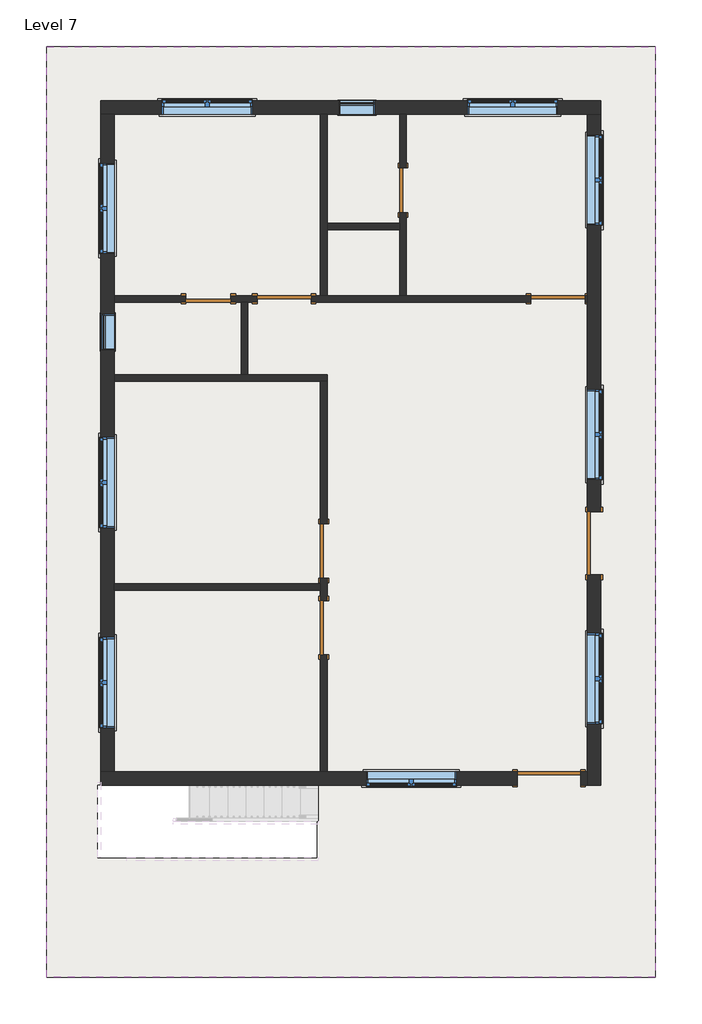
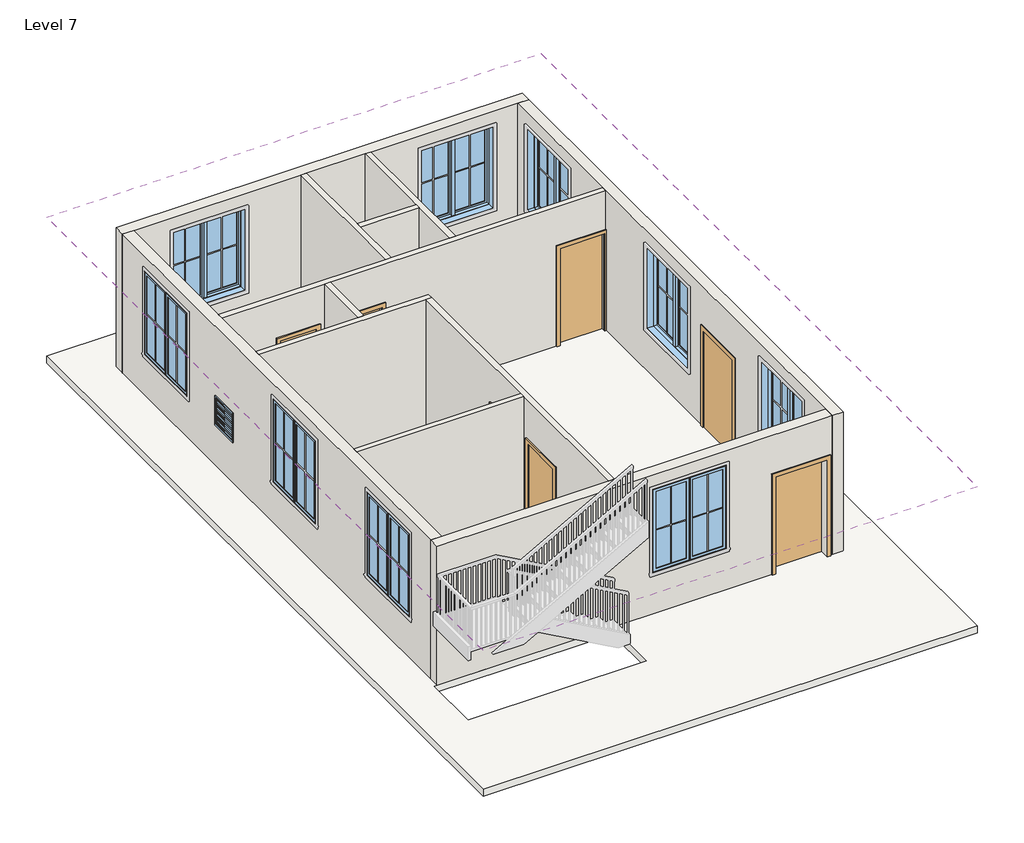
# One storey, part 1 of 3: 12 walls, 11 windows, 8 doors, 2 roofs.
"""IFC4 building model written with IfcOpenShell, lengths in millimetres."""

from ifc_helpers import new_model, si_unit, frame, origin, place, context, project, spatial, polyline, outline, extrude, faceted_brep, transform, mapped, element, save
from components import door_78caadf7, single_flush_door_3_e5f9f3c4, single_flush_door_3_305aa2a5, door_9d399b00, door_0848dd25, window_casement_double_win_5_f93960c7, window_f2d8fef0

model = new_model("IFC4")

# Units and contexts
model_context = context("Model", 3, world=origin())
ifc_project = project(units=[si_unit("LENGTHUNIT", "METRE", prefix="MILLI")], contexts=[model_context])

# Site, building, storey
site = spatial("IfcSite", under=ifc_project)
building = spatial("IfcBuilding", under=site)
storey = spatial("IfcBuildingStorey", under=building, Name="Level 7", Elevation=16002.0)

# Doors
placement = place(None, origin())
door_shape = door_78caadf7(model_context)
element("IfcDoor", 1, ObjectType="Single-Flush : DOOR 2'6\"", at=placement, inside=storey, context=model_context, shape_type="MappedRepresentation", body=[
    mapped(door_shape, transform((-377.1698569, 4707.5566963, 16002.0), x_axis=(0.0, -1.0, 0.0), y_axis=(1.0, 0.0, 0.0), z_axis=(0.0, 0.0, 1.0))),
])
element("IfcDoor", 2, ObjectType="Single-Flush : DOOR 2'6\"", at=placement, inside=storey, context=model_context, shape_type="MappedRepresentation", body=[
    mapped(door_shape, transform((-3653.7698569, 2878.7566963, 16002.0), x_axis=(1.0, 0.0, 0.0), y_axis=(0.0, 1.0, 0.0), z_axis=(0.0, 0.0, 1.0))),
])
single_flush_door_3_shape = single_flush_door_3_e5f9f3c4(model_context)
element("IfcDoor", 3, ObjectType="Single-Flush : DOOR 3'", at=placement, inside=storey, context=model_context, shape_type="MappedRepresentation", body=[
    mapped(single_flush_door_3_shape, transform((-2377.4198569, 2878.7566963, 16002.0), x_axis=(1.0, 0.0, 0.0), y_axis=(0.0, 1.0, 0.0), z_axis=(0.0, 0.0, 1.0))),
])
element("IfcDoor", 4, ObjectType="Single-Flush : DOOR 3'", at=placement, inside=storey, context=model_context, shape_type="MappedRepresentation", body=[
    mapped(single_flush_door_3_shape, transform((2232.6801431, 2878.7566963, 16002.0), x_axis=(1.0, 0.0, 0.0), y_axis=(0.0, 1.0, 0.0), z_axis=(0.0, 0.0, 1.0))),
])
element("IfcDoor", 5, ObjectType="Single-Flush : DOOR 3'", at=placement, inside=storey, context=model_context, shape_type="MappedRepresentation", body=[
    mapped(single_flush_door_3_shape, transform((-1710.6698569, -2658.4433037, 16002.0), x_axis=(0.0, 1.0, 0.0), y_axis=(-1.0, 0.0, 0.0), z_axis=(0.0, 0.0, 1.0))),
])
single_flush_door_3_2_shape = single_flush_door_3_305aa2a5(model_context)
element("IfcDoor", 6, ObjectType="Single-Flush : DOOR 3'", at=placement, inside=storey, context=model_context, shape_type="MappedRepresentation", body=[
    mapped(single_flush_door_3_2_shape, transform((-1710.6698569, -1363.0433037, 16002.0), x_axis=(0.0, -1.0, 0.0), y_axis=(1.0, 0.0, 0.0), z_axis=(0.0, 0.0, 1.0))),
])
door_2_shape = door_9d399b00(model_context)
element("IfcDoor", 7, ObjectType="Single-Flush : DOOR 3'6\"", at=placement, inside=storey, context=model_context, shape_type="MappedRepresentation", body=[
    mapped(door_2_shape, transform((2080.2801431, -5192.0933037, 16002.0), x_axis=(1.0, 0.0, 0.0), y_axis=(0.0, 1.0, 0.0), z_axis=(0.0, 0.0, 1.0))),
])
door_3_shape = door_0848dd25(model_context)
element("IfcDoor", 8, ObjectType="Single-Flush : DOOR 3'6\"", at=placement, inside=storey, context=model_context, shape_type="MappedRepresentation", body=[
    mapped(door_3_shape, transform((2842.2801431, -1236.0433037, 16002.0), x_axis=(0.0, -1.0, 0.0), y_axis=(1.0, 0.0, 0.0), z_axis=(0.0, 0.0, 1.0))),
])

# Roofs
element("IfcRoof", 9, ObjectType="ROOF 6\"", at=placement, inside=storey, context=model_context, shape_type="SweptSolid", body=[
    extrude(outline(polyline([(-6377.9198569, -8544.8933037), (-6377.9198569, 7126.9066963), (3870.9801431, 7126.9066963), (3870.9801431, -8544.8933037), (-6377.9198569, -8544.8933037)]), holes=[polyline([(-5514.3198569, -5306.3933037), (-5514.3198569, -6525.5933037), (-1831.3198569, -6525.5933037), (-1831.3198569, -5306.3933037), (-5514.3198569, -5306.3933037)])]), frame((0.0, 0.0, 15849.6), z_axis=(0.0, 0.0, 1.0), x_axis=(1.0, 0.0, 0.0)), (0.0, 0.0, 1.0), 152.4),
])
element("IfcRoof", 10, ObjectType="ROOF 6\"", at=placement, inside=storey, context=model_context, shape_type="SweptSolid", body=[
    extrude(outline(polyline([(-6377.9198569, -8544.8933037), (-6377.9198569, 7126.9066963), (3870.9801431, 7126.9066963), (3870.9801431, -8544.8933037), (-6377.9198569, -8544.8933037)]), holes=[polyline([(-5514.3198569, -5306.3933037), (-5514.3198569, -6525.5933037), (-1831.3198569, -6525.5933037), (-1831.3198569, -5306.3933037), (-5514.3198569, -5306.3933037)])]), frame((0.0, 0.0, 19050.0), z_axis=(0.0, 0.0, 1.0), x_axis=(1.0, 0.0, 0.0)), (0.0, 0.0, 1.0), 152.4),
])

# Walls
element("IfcWall", 11, ObjectType="WALL 4.5\"", at=placement, inside=storey, context=model_context, shape_type="Brep", body=[
    faceted_brep([(2689.8801431, 2821.6066963, 18135.6), (2689.8801431, 2821.6066963, 16002.0), (2727.9801431, 2821.6066963, 16002.0), (2727.9801431, 2821.6066963, 19050.0), (-2987.0198569, 2821.6066963, 19050.0), (-3101.3198569, 2821.6066963, 19050.0), (-5234.9198569, 2821.6066963, 19050.0), (-5234.9198569, 2821.6066963, 16002.0), (-4034.7698569, 2821.6066963, 16002.0), (-4034.7698569, 2821.6066963, 18135.6), (-3272.7698569, 2821.6066963, 18135.6), (-3272.7698569, 2821.6066963, 16002.0), (-3101.3198569, 2821.6066963, 16002.0), (-2987.0198569, 2821.6066963, 16002.0), (-2834.6198569, 2821.6066963, 16002.0), (-2834.6198569, 2821.6066963, 18135.6), (-1920.2198569, 2821.6066963, 18135.6), (-1920.2198569, 2821.6066963, 16002.0), (1775.4801431, 2821.6066963, 16002.0), (1775.4801431, 2821.6066963, 18135.6), (2727.9801431, 2935.9066963, 16002.0), (2689.8801431, 2935.9066963, 16002.0), (2689.8801431, 2935.9066963, 18135.6), (1775.4801431, 2935.9066963, 18135.6), (1775.4801431, 2935.9066963, 16002.0), (-320.0198569, 2935.9066963, 16002.0), (-434.3198569, 2935.9066963, 16002.0), (-1653.5198569, 2935.9066963, 16002.0), (-1767.8198569, 2935.9066963, 16002.0), (-1920.2198569, 2935.9066963, 16002.0), (-1920.2198569, 2935.9066963, 18135.6), (-2834.6198569, 2935.9066963, 18135.6), (-2834.6198569, 2935.9066963, 16002.0), (-3272.7698569, 2935.9066963, 16002.0), (-3272.7698569, 2935.9066963, 18135.6), (-4034.7698569, 2935.9066963, 18135.6), (-4034.7698569, 2935.9066963, 16002.0), (-5234.9198569, 2935.9066963, 16002.0), (-5234.9198569, 2935.9066963, 19050.0), (-1767.8198569, 2935.9066963, 19050.0), (-1653.5198569, 2935.9066963, 19050.0), (-434.3198569, 2935.9066963, 19050.0), (-320.0198569, 2935.9066963, 19050.0), (2727.9801431, 2935.9066963, 19050.0)], [[[0, 1, 2, 3, 4, 5, 6, 7, 8, 9, 10, 11, 12, 13, 14, 15, 16, 17, 18, 19]], [[20, 21, 22, 23, 24, 25, 26, 27, 28, 29, 30, 31, 32, 33, 34, 35, 36, 37, 38, 39, 40, 41, 42, 43]], [[8, 7, 37, 36]], [[14, 13, 12, 11, 33, 32]], [[18, 17, 29, 28, 27, 26, 25, 24]], [[2, 1, 21, 20]], [[3, 2, 20, 43]], [[7, 6, 38, 37]], [[34, 33, 11, 10]], [[35, 34, 10, 9]], [[36, 35, 9, 8]], [[30, 29, 17, 16]], [[31, 30, 16, 15]], [[32, 31, 15, 14]], [[22, 21, 1, 0]], [[23, 22, 0, 19]], [[24, 23, 19, 18]], [[6, 5, 4, 3, 43, 42, 41, 40, 39, 38]]]),
])
element("IfcWall", 12, ObjectType="WALL 4.5\"", at=placement, inside=storey, context=model_context, shape_type="Brep", body=[
    faceted_brep([(-1767.8198569, 5983.9066963, 16002.0), (-1767.8198569, 2935.9066963, 16002.0), (-1767.8198569, 2935.9066963, 19050.0), (-1767.8198569, 5983.9066963, 19050.0), (-1653.5198569, 5983.9066963, 16002.0), (-1653.5198569, 5983.9066963, 19050.0), (-1653.5198569, 4155.1066963, 19050.0), (-1653.5198569, 4040.8066963, 19050.0), (-1653.5198569, 2935.9066963, 19050.0), (-1653.5198569, 2935.9066963, 16002.0), (-1653.5198569, 4040.8066963, 16002.0), (-1653.5198569, 4155.1066963, 16002.0)], [[[0, 1, 2, 3]], [[4, 5, 6, 7, 8, 9, 10, 11]], [[1, 0, 4, 11, 10, 9]], [[0, 3, 5, 4]], [[2, 1, 9, 8]], [[3, 2, 8, 7, 6, 5]]]),
])
element("IfcWall", 13, ObjectType="WALL 4.5\"", at=placement, inside=storey, context=model_context, shape_type="Brep", body=[
    faceted_brep([(-320.0198569, 2935.9066963, 16002.0), (-320.0198569, 4326.5566963, 16002.0), (-320.0198569, 4326.5566963, 18135.6), (-320.0198569, 5088.5566963, 18135.6), (-320.0198569, 5088.5566963, 16002.0), (-320.0198569, 5983.9066963, 16002.0), (-320.0198569, 5983.9066963, 19050.0), (-320.0198569, 2935.9066963, 19050.0), (-434.3198569, 4326.5566963, 18135.6), (-434.3198569, 4326.5566963, 16002.0), (-434.3198569, 4155.1066963, 16002.0), (-434.3198569, 4040.8066963, 16002.0), (-434.3198569, 2935.9066963, 16002.0), (-434.3198569, 2935.9066963, 19050.0), (-434.3198569, 4040.8066963, 19050.0), (-434.3198569, 4155.1066963, 19050.0), (-434.3198569, 5983.9066963, 19050.0), (-434.3198569, 5983.9066963, 16002.0), (-434.3198569, 5088.5566963, 16002.0), (-434.3198569, 5088.5566963, 18135.6)], [[[0, 1, 2, 3, 4, 5, 6, 7]], [[8, 9, 10, 11, 12, 13, 14, 15, 16, 17, 18, 19]], [[18, 17, 5, 4]], [[12, 11, 10, 9, 1, 0]], [[6, 5, 17, 16]], [[0, 7, 13, 12]], [[2, 1, 9, 8]], [[3, 2, 8, 19]], [[4, 3, 19, 18]], [[7, 6, 16, 15, 14, 13]]]),
])
element("IfcWall", 14, ObjectType="WALL 4.5\"", at=placement, inside=storey, context=model_context, shape_type="SweptSolid", body=[
    extrude(outline(polyline([(-434.3198569, 4040.8066963), (-1653.5198569, 4040.8066963), (-1653.5198569, 4155.1066963), (-434.3198569, 4155.1066963), (-434.3198569, 4040.8066963)])), frame((0.0, 0.0, 16002.0), z_axis=(0.0, 0.0, 1.0), x_axis=(1.0, 0.0, 0.0)), (0.0, 0.0, 1.0), 3048.0),
])
element("IfcWall", 15, ObjectType="WALL 4.5\"", at=placement, inside=storey, context=model_context, shape_type="Brep", body=[
    faceted_brep([(-5234.9198569, 1488.1066963, 16002.0), (-1767.8198569, 1488.1066963, 16002.0), (-1653.5198569, 1488.1066963, 16002.0), (-1653.5198569, 1488.1066963, 19050.0), (-1767.8198569, 1488.1066963, 19050.0), (-5234.9198569, 1488.1066963, 19050.0), (-5234.9198569, 1602.4066963, 16002.0), (-5234.9198569, 1602.4066963, 19050.0), (-3101.3198569, 1602.4066963, 19050.0), (-2987.0198569, 1602.4066963, 19050.0), (-1653.5198569, 1602.4066963, 19050.0), (-1653.5198569, 1602.4066963, 16002.0), (-2987.0198569, 1602.4066963, 16002.0), (-3101.3198569, 1602.4066963, 16002.0)], [[[0, 1, 2, 3, 4, 5]], [[6, 7, 8, 9, 10, 11, 12, 13]], [[2, 1, 0, 6, 13, 12, 11]], [[0, 5, 7, 6]], [[3, 2, 11, 10]], [[5, 4, 3, 10, 9, 8, 7]]]),
])
element("IfcWall", 16, ObjectType="WALL 4.5\"", at=placement, inside=storey, context=model_context, shape_type="Brep", body=[
    faceted_brep([(-1767.8198569, -1820.2433037, 16002.0), (-1767.8198569, -1915.4933037, 16002.0), (-1767.8198569, -2029.7933037, 16002.0), (-1767.8198569, -2201.2433037, 16002.0), (-1767.8198569, -2201.2433037, 18135.6), (-1767.8198569, -3115.6433037, 18135.6), (-1767.8198569, -3115.6433037, 16002.0), (-1767.8198569, -5077.7933037, 16002.0), (-1767.8198569, -5077.7933037, 19050.0), (-1767.8198569, -2029.7933037, 19050.0), (-1767.8198569, -1915.4933037, 19050.0), (-1767.8198569, 1488.1066963, 19050.0), (-1767.8198569, 1488.1066963, 16002.0), (-1767.8198569, -905.8433037, 16002.0), (-1767.8198569, -905.8433037, 18135.6), (-1767.8198569, -1820.2433037, 18135.6), (-1653.5198569, -2201.2433037, 18135.6), (-1653.5198569, -2201.2433037, 16002.0), (-1653.5198569, -1820.2433037, 16002.0), (-1653.5198569, -1820.2433037, 18135.6), (-1653.5198569, -905.8433037, 18135.6), (-1653.5198569, -905.8433037, 16002.0), (-1653.5198569, 1488.1066963, 16002.0), (-1653.5198569, 1488.1066963, 19050.0), (-1653.5198569, -5077.7933037, 19050.0), (-1653.5198569, -5077.7933037, 16002.0), (-1653.5198569, -3115.6433037, 16002.0), (-1653.5198569, -3115.6433037, 18135.6)], [[[0, 1, 2, 3, 4, 5, 6, 7, 8, 9, 10, 11, 12, 13, 14, 15]], [[16, 17, 18, 19, 20, 21, 22, 23, 24, 25, 26, 27]], [[13, 12, 22, 21]], [[26, 25, 7, 6]], [[18, 17, 3, 2, 1, 0]], [[12, 11, 23, 22]], [[8, 7, 25, 24]], [[19, 18, 0, 15]], [[20, 19, 15, 14]], [[21, 20, 14, 13]], [[4, 3, 17, 16]], [[5, 4, 16, 27]], [[6, 5, 27, 26]], [[11, 10, 9, 8, 24, 23]]]),
])
element("IfcWall", 17, ObjectType="WALL 4.5\"", at=placement, inside=storey, context=model_context, shape_type="SweptSolid", body=[
    extrude(outline(polyline([(-1767.8198569, -2029.7933037), (-5234.9198569, -2029.7933037), (-5234.9198569, -1915.4933037), (-1767.8198569, -1915.4933037), (-1767.8198569, -2029.7933037)])), frame((0.0, 0.0, 16002.0), z_axis=(0.0, 0.0, 1.0), x_axis=(1.0, 0.0, 0.0)), (0.0, 0.0, 1.0), 3048.0),
])
element("IfcWall", 18, ObjectType="WALL 4.5\"", at=placement, inside=storey, context=model_context, shape_type="SweptSolid", body=[
    extrude(outline(polyline([(-3101.3198569, 1602.4066963), (-3101.3198569, 2821.6066963), (-2987.0198569, 2821.6066963), (-2987.0198569, 1602.4066963), (-3101.3198569, 1602.4066963)])), frame((0.0, 0.0, 16002.0), z_axis=(0.0, 0.0, 1.0), x_axis=(1.0, 0.0, 0.0)), (0.0, 0.0, 1.0), 3048.0),
])
element("IfcWall", 19, ObjectType="WALL 9\"", at=placement, inside=storey, context=model_context, shape_type="Brep", body=[
    faceted_brep([(-5463.5198569, 5983.9066963, 16002.0), (-5234.9198569, 5983.9066963, 16002.0), (-1767.8198569, 5983.9066963, 16002.0), (-1653.5198569, 5983.9066963, 16002.0), (-434.3198569, 5983.9066963, 16002.0), (-320.0198569, 5983.9066963, 16002.0), (2727.9801431, 5983.9066963, 16002.0), (2956.5801431, 5983.9066963, 16002.0), (2956.5801431, 5983.9066963, 19050.0), (2727.9801431, 5983.9066963, 19050.0), (-320.0198569, 5983.9066963, 19050.0), (-434.3198569, 5983.9066963, 19050.0), (-1653.5198569, 5983.9066963, 19050.0), (-1767.8198569, 5983.9066963, 19050.0), (-5234.9198569, 5983.9066963, 19050.0), (-5463.5198569, 5983.9066963, 19050.0), (2232.6801431, 5983.9066963, 18745.2), (2232.6801431, 5983.9066963, 16916.4), (708.6801431, 5983.9066963, 16916.4), (708.6801431, 5983.9066963, 18745.2), (-2910.8198569, 5983.9066963, 18745.2), (-2910.8198569, 5983.9066963, 16916.4), (-4434.8198569, 5983.9066963, 16916.4), (-4434.8198569, 5983.9066963, 18745.2), (-1456.6698569, 5983.9066963, 17526.0), (-847.0698569, 5983.9066963, 17526.0), (-847.0698569, 5983.9066963, 16916.4), (-1456.6698569, 5983.9066963, 16916.4), (-5463.5198569, 6212.5066963, 16002.0), (-5463.5198569, 6212.5066963, 19050.0), (2956.5801431, 6212.5066963, 19050.0), (2956.5801431, 6212.5066963, 16002.0), (2232.6801431, 6212.5066963, 18745.2), (708.6801431, 6212.5066963, 18745.2), (708.6801431, 6212.5066963, 16916.4), (2232.6801431, 6212.5066963, 16916.4), (-2910.8198569, 6212.5066963, 18745.2), (-4434.8198569, 6212.5066963, 18745.2), (-4434.8198569, 6212.5066963, 16916.4), (-2910.8198569, 6212.5066963, 16916.4), (-1456.6698569, 6212.5066963, 17526.0), (-1456.6698569, 6212.5066963, 16916.4), (-847.0698569, 6212.5066963, 16916.4), (-847.0698569, 6212.5066963, 17526.0)], [[[0, 1, 2, 3, 4, 5, 6, 7, 8, 9, 10, 11, 12, 13, 14, 15], [16, 17, 18, 19], [20, 21, 22, 23], [24, 25, 26, 27]], [[28, 29, 30, 31], [32, 33, 34, 35], [36, 37, 38, 39], [40, 41, 42, 43]], [[7, 6, 5, 4, 3, 2, 1, 0, 28, 31]], [[8, 7, 31, 30]], [[0, 15, 29, 28]], [[17, 16, 32, 35]], [[18, 17, 35, 34]], [[19, 18, 34, 33]], [[16, 19, 33, 32]], [[21, 20, 36, 39]], [[22, 21, 39, 38]], [[23, 22, 38, 37]], [[20, 23, 37, 36]], [[41, 40, 24, 27]], [[42, 41, 27, 26]], [[43, 42, 26, 25]], [[40, 43, 25, 24]], [[15, 14, 13, 12, 11, 10, 9, 8, 30, 29]]]),
])
element("IfcWall", 20, ObjectType="WALL 9\"", at=placement, inside=storey, context=model_context, shape_type="Brep", body=[
    faceted_brep([(2727.9801431, -1769.4433037, 18135.6), (2727.9801431, -1769.4433037, 16002.0), (2727.9801431, -5077.7933037, 16002.0), (2727.9801431, -5306.3933037, 16002.0), (2727.9801431, -5306.3933037, 19050.0), (2727.9801431, -5077.7933037, 19050.0), (2727.9801431, 2821.6066963, 19050.0), (2727.9801431, 2935.9066963, 19050.0), (2727.9801431, 5983.9066963, 19050.0), (2727.9801431, 5983.9066963, 16002.0), (2727.9801431, 2935.9066963, 16002.0), (2727.9801431, 2821.6066963, 16002.0), (2727.9801431, -702.6433037, 16002.0), (2727.9801431, -702.6433037, 18135.6), (2727.9801431, 4117.0066963, 18745.2), (2727.9801431, 4117.0066963, 16916.4), (2727.9801431, 5641.0066963, 16916.4), (2727.9801431, 5641.0066963, 18745.2), (2727.9801431, -169.2433037, 18745.2), (2727.9801431, -169.2433037, 16916.4), (2727.9801431, 1354.7566963, 16916.4), (2727.9801431, 1354.7566963, 18745.2), (2727.9801431, -4277.6933037, 18745.2), (2727.9801431, -4277.6933037, 16916.4), (2727.9801431, -2753.6933037, 16916.4), (2727.9801431, -2753.6933037, 18745.2), (2956.5801431, -5306.3933037, 16002.0), (2956.5801431, -1769.4433037, 16002.0), (2956.5801431, -1769.4433037, 18135.6), (2956.5801431, -702.6433037, 18135.6), (2956.5801431, -702.6433037, 16002.0), (2956.5801431, 5983.9066963, 16002.0), (2956.5801431, 5983.9066963, 19050.0), (2956.5801431, -5306.3933037, 19050.0), (2956.5801431, 4117.0066963, 18745.2), (2956.5801431, 5641.0066963, 18745.2), (2956.5801431, 5641.0066963, 16916.4), (2956.5801431, 4117.0066963, 16916.4), (2956.5801431, -169.2433037, 18745.2), (2956.5801431, 1354.7566963, 18745.2), (2956.5801431, 1354.7566963, 16916.4), (2956.5801431, -169.2433037, 16916.4), (2956.5801431, -4277.6933037, 18745.2), (2956.5801431, -2753.6933037, 18745.2), (2956.5801431, -2753.6933037, 16916.4), (2956.5801431, -4277.6933037, 16916.4)], [[[0, 1, 2, 3, 4, 5, 6, 7, 8, 9, 10, 11, 12, 13], [14, 15, 16, 17], [18, 19, 20, 21], [22, 23, 24, 25]], [[26, 27, 28, 29, 30, 31, 32, 33], [34, 35, 36, 37], [38, 39, 40, 41], [42, 43, 44, 45]], [[3, 2, 1, 27, 26]], [[12, 11, 10, 9, 31, 30]], [[9, 8, 32, 31]], [[4, 3, 26, 33]], [[15, 14, 34, 37]], [[16, 15, 37, 36]], [[17, 16, 36, 35]], [[14, 17, 35, 34]], [[19, 18, 38, 41]], [[20, 19, 41, 40]], [[21, 20, 40, 39]], [[18, 21, 39, 38]], [[23, 22, 42, 45]], [[24, 23, 45, 44]], [[25, 24, 44, 43]], [[22, 25, 43, 42]], [[28, 27, 1, 0]], [[29, 28, 0, 13]], [[30, 29, 13, 12]], [[8, 7, 6, 5, 4, 33, 32]]]),
])
element("IfcWall", 21, ObjectType="WALL 9\"", at=placement, inside=storey, context=model_context, shape_type="Brep", body=[
    faceted_brep([(2727.9801431, -5077.7933037, 16002.0), (2613.6801431, -5077.7933037, 16002.0), (2613.6801431, -5077.7933037, 18135.6), (1546.8801431, -5077.7933037, 18135.6), (1546.8801431, -5077.7933037, 16002.0), (-1653.5198569, -5077.7933037, 16002.0), (-1767.8198569, -5077.7933037, 16002.0), (-5234.9198569, -5077.7933037, 16002.0), (-5463.5198569, -5077.7933037, 16002.0), (-5463.5198569, -5077.7933037, 19050.0), (-5234.9198569, -5077.7933037, 19050.0), (-1767.8198569, -5077.7933037, 19050.0), (-1653.5198569, -5077.7933037, 19050.0), (2727.9801431, -5077.7933037, 19050.0), (-999.4698569, -5077.7933037, 18745.2), (-999.4698569, -5077.7933037, 16916.4), (524.5301431, -5077.7933037, 16916.4), (524.5301431, -5077.7933037, 18745.2), (2613.6801431, -5306.3933037, 18135.6), (2613.6801431, -5306.3933037, 16002.0), (2727.9801431, -5306.3933037, 16002.0), (2727.9801431, -5306.3933037, 19050.0), (-1831.3198569, -5306.3933037, 19050.0), (-5463.5198569, -5306.3933037, 19050.0), (-5463.5198569, -5306.3933037, 16002.0), (1546.8801431, -5306.3933037, 16002.0), (1546.8801431, -5306.3933037, 18135.6), (-999.4698569, -5306.3933037, 18745.2), (524.5301431, -5306.3933037, 18745.2), (524.5301431, -5306.3933037, 16916.4), (-999.4698569, -5306.3933037, 16916.4)], [[[0, 1, 2, 3, 4, 5, 6, 7, 8, 9, 10, 11, 12, 13], [14, 15, 16, 17]], [[18, 19, 20, 21, 22, 23, 24, 25, 26], [27, 28, 29, 30]], [[25, 24, 8, 7, 6, 5, 4]], [[20, 19, 1, 0]], [[0, 13, 21, 20]], [[9, 8, 24, 23]], [[15, 14, 27, 30]], [[16, 15, 30, 29]], [[17, 16, 29, 28]], [[14, 17, 28, 27]], [[2, 1, 19, 18]], [[3, 2, 18, 26]], [[4, 3, 26, 25]], [[13, 12, 11, 10, 9, 23, 22, 21]]]),
])
element("IfcWall", 22, ObjectType="WALL 9\"", at=placement, inside=storey, context=model_context, shape_type="Brep", body=[
    faceted_brep([(-5234.9198569, -5077.7933037, 16002.0), (-5234.9198569, -2029.7933037, 16002.0), (-5234.9198569, -1915.4933037, 16002.0), (-5234.9198569, 1488.1066963, 16002.0), (-5234.9198569, 1602.4066963, 16002.0), (-5234.9198569, 2821.6066963, 16002.0), (-5234.9198569, 2935.9066963, 16002.0), (-5234.9198569, 5983.9066963, 16002.0), (-5234.9198569, 5983.9066963, 19050.0), (-5234.9198569, 2935.9066963, 19050.0), (-5234.9198569, 2821.6066963, 19050.0), (-5234.9198569, 1602.4066963, 19050.0), (-5234.9198569, 1488.1066963, 19050.0), (-5234.9198569, -1915.4933037, 19050.0), (-5234.9198569, -2029.7933037, 19050.0), (-5234.9198569, -5077.7933037, 19050.0), (-5234.9198569, -2820.3683037, 18745.2), (-5234.9198569, -2820.3683037, 16916.4), (-5234.9198569, -4344.3683037, 16916.4), (-5234.9198569, -4344.3683037, 18745.2), (-5234.9198569, 548.3066963, 18745.2), (-5234.9198569, 548.3066963, 16916.4), (-5234.9198569, -975.6933037, 16916.4), (-5234.9198569, -975.6933037, 18745.2), (-5234.9198569, 5164.7566963, 18745.2), (-5234.9198569, 5164.7566963, 16916.4), (-5234.9198569, 3640.7566963, 16916.4), (-5234.9198569, 3640.7566963, 18745.2), (-5234.9198569, 2015.1566963, 17526.0), (-5234.9198569, 2624.7566963, 17526.0), (-5234.9198569, 2624.7566963, 16916.4), (-5234.9198569, 2015.1566963, 16916.4), (-5463.5198569, -5077.7933037, 16002.0), (-5463.5198569, -5077.7933037, 19050.0), (-5463.5198569, 5983.9066963, 19050.0), (-5463.5198569, 5983.9066963, 16002.0), (-5463.5198569, -2820.3683037, 18745.2), (-5463.5198569, -4344.3683037, 18745.2), (-5463.5198569, -4344.3683037, 16916.4), (-5463.5198569, -2820.3683037, 16916.4), (-5463.5198569, 548.3066963, 18745.2), (-5463.5198569, -975.6933037, 18745.2), (-5463.5198569, -975.6933037, 16916.4), (-5463.5198569, 548.3066963, 16916.4), (-5463.5198569, 5164.7566963, 18745.2), (-5463.5198569, 3640.7566963, 18745.2), (-5463.5198569, 3640.7566963, 16916.4), (-5463.5198569, 5164.7566963, 16916.4), (-5463.5198569, 2015.1566963, 17526.0), (-5463.5198569, 2015.1566963, 16916.4), (-5463.5198569, 2624.7566963, 16916.4), (-5463.5198569, 2624.7566963, 17526.0)], [[[0, 1, 2, 3, 4, 5, 6, 7, 8, 9, 10, 11, 12, 13, 14, 15], [16, 17, 18, 19], [20, 21, 22, 23], [24, 25, 26, 27], [28, 29, 30, 31]], [[32, 33, 34, 35], [36, 37, 38, 39], [40, 41, 42, 43], [44, 45, 46, 47], [48, 49, 50, 51]], [[7, 6, 5, 4, 3, 2, 1, 0, 32, 35]], [[8, 7, 35, 34]], [[0, 15, 33, 32]], [[17, 16, 36, 39]], [[18, 17, 39, 38]], [[19, 18, 38, 37]], [[16, 19, 37, 36]], [[21, 20, 40, 43]], [[22, 21, 43, 42]], [[23, 22, 42, 41]], [[20, 23, 41, 40]], [[25, 24, 44, 47]], [[26, 25, 47, 46]], [[27, 26, 46, 45]], [[24, 27, 45, 44]], [[49, 48, 28, 31]], [[50, 49, 31, 30]], [[51, 50, 30, 29]], [[48, 51, 29, 28]], [[15, 14, 13, 12, 11, 10, 9, 8, 34, 33]]]),
])

# Windows
window_casement_double_win_5_shape = window_casement_double_win_5_f93960c7(model_context)
element("IfcWindow", 23, ObjectType="Window-Casement-Double : WIN 5'", at=placement, inside=storey, context=model_context, shape_type="MappedRepresentation", body=[
    mapped(window_casement_double_win_5_shape, transform((-5349.2198569, -3582.3683037, 16002.0), x_axis=(0.0, 1.0, 0.0), y_axis=(-1.0, 0.0, 0.0), z_axis=(0.0, 0.0, 1.0))),
])
element("IfcWindow", 24, ObjectType="Window-Casement-Double : WIN 5'", at=placement, inside=storey, context=model_context, shape_type="MappedRepresentation", body=[
    mapped(window_casement_double_win_5_shape, transform((-5349.2198569, -213.6933037, 16002.0), x_axis=(0.0, 1.0, 0.0), y_axis=(-1.0, 0.0, 0.0), z_axis=(0.0, 0.0, 1.0))),
])
element("IfcWindow", 25, ObjectType="Window-Casement-Double : WIN 5'", at=placement, inside=storey, context=model_context, shape_type="MappedRepresentation", body=[
    mapped(window_casement_double_win_5_shape, transform((-5349.2198569, 4402.7566963, 16002.0), x_axis=(0.0, 1.0, 0.0), y_axis=(-1.0, 0.0, 0.0), z_axis=(0.0, 0.0, 1.0))),
])
element("IfcWindow", 26, ObjectType="Window-Casement-Double : WIN 5'", at=placement, inside=storey, context=model_context, shape_type="MappedRepresentation", body=[
    mapped(window_casement_double_win_5_shape, transform((2842.2801431, 4879.0066963, 16002.0), x_axis=(0.0, -1.0, 0.0), y_axis=(1.0, 0.0, 0.0), z_axis=(0.0, 0.0, 1.0))),
])
element("IfcWindow", 27, ObjectType="Window-Casement-Double : WIN 5'", at=placement, inside=storey, context=model_context, shape_type="MappedRepresentation", body=[
    mapped(window_casement_double_win_5_shape, transform((2842.2801431, 592.7566963, 16002.0), x_axis=(0.0, -1.0, 0.0), y_axis=(1.0, 0.0, 0.0), z_axis=(0.0, 0.0, 1.0))),
])
element("IfcWindow", 28, ObjectType="Window-Casement-Double : WIN 5'", at=placement, inside=storey, context=model_context, shape_type="MappedRepresentation", body=[
    mapped(window_casement_double_win_5_shape, transform((2842.2801431, -3515.6933037, 16002.0), x_axis=(0.0, -1.0, 0.0), y_axis=(1.0, 0.0, 0.0), z_axis=(0.0, 0.0, 1.0))),
])
element("IfcWindow", 29, ObjectType="Window-Casement-Double : WIN 5'", at=placement, inside=storey, context=model_context, shape_type="MappedRepresentation", body=[
    mapped(window_casement_double_win_5_shape, transform((-237.4698569, -5192.0933037, 16002.0), x_axis=(-1.0, 0.0, 0.0), y_axis=(0.0, -1.0, 0.0), z_axis=(0.0, 0.0, 1.0))),
])
element("IfcWindow", 30, ObjectType="Window-Casement-Double : WIN 5'", at=placement, inside=storey, context=model_context, shape_type="MappedRepresentation", body=[
    mapped(window_casement_double_win_5_shape, transform((1470.6801431, 6098.2066963, 16002.0), x_axis=(1.0, 0.0, 0.0), y_axis=(0.0, 1.0, 0.0), z_axis=(0.0, 0.0, 1.0))),
])
element("IfcWindow", 31, ObjectType="Window-Casement-Double : WIN 5'", at=placement, inside=storey, context=model_context, shape_type="MappedRepresentation", body=[
    mapped(window_casement_double_win_5_shape, transform((-3672.8198569, 6098.2066963, 16002.0), x_axis=(1.0, 0.0, 0.0), y_axis=(0.0, 1.0, 0.0), z_axis=(0.0, 0.0, 1.0))),
])
window_shape = window_f2d8fef0(model_context)
element("IfcWindow", 32, ObjectType="Window-Louvers : 24\" x 24\"", at=placement, inside=storey, context=model_context, shape_type="MappedRepresentation", body=[
    mapped(window_shape, transform((-1151.8698569, 6104.5566963, 16002.0), x_axis=(1.0, 0.0, 0.0), y_axis=(0.0, 1.0, 0.0), z_axis=(0.0, 0.0, 1.0))),
])
element("IfcWindow", 33, ObjectType="Window-Louvers : 24\" x 24\"", at=placement, inside=storey, context=model_context, shape_type="MappedRepresentation", body=[
    mapped(window_shape, transform((-5355.5698569, 2319.9566963, 16002.0), x_axis=(0.0, 1.0, 0.0), y_axis=(-1.0, 0.0, 0.0), z_axis=(0.0, 0.0, 1.0))),
])

save(model, "model.ifc")

# Revit data of these elements
# Type "Single-Flush : DOOR 2'6\""
#   Type Mark = "10"
#   Construction Type Id = "MDOOR"
#   Assembly Code = "C1020"
#   Analytic Construction = "Metal"
#   Thickness = 0' - 2"
#   Heat Transfer Coefficient (U) = 0.651978 BTU/(h·ft²·°F)
#   Height = 7' - 0"
#   Trim Projection Ext = 0' - 1"
#   Trim Projection Int = 0' - 1"
#   Trim Width = 0' - 3"
#   Width = 2' - 6"
#   Define Thermal Properties by = 1
#   Door Material = Door - Panel
#   Frame Material = Door - Frame
#   Visual Light Transmittance = 0
#   Solar Heat Gain Coefficient = 0
#   Function = (empty or 0)
#   Wall Closure = (empty or 0)
# Type "Single-Flush : DOOR 3'"
#   Type Mark = "8"
#   Construction Type Id = "MDOOR"
#   Assembly Code = "C1020"
#   Analytic Construction = "Metal"
#   Thickness = 0' - 2"
#   Heat Transfer Coefficient (U) = 0.651978 BTU/(h·ft²·°F)
#   Height = 7' - 0"
#   Trim Projection Ext = 0' - 1"
#   Trim Projection Int = 0' - 1"
#   Trim Width = 0' - 3"
#   Width = 3' - 0"
#   Define Thermal Properties by = 1
#   Door Material = Door - Panel
#   Frame Material = Door - Frame
#   Visual Light Transmittance = 0
#   Solar Heat Gain Coefficient = 0
#   Function = (empty or 0)
#   Wall Closure = (empty or 0)
# Type "Single-Flush : DOOR 3'6\""
#   Type Mark = "9"
#   Construction Type Id = "MDOOR"
#   Assembly Code = "C1020"
#   Analytic Construction = "Metal"
#   Thickness = 0' - 2"
#   Heat Transfer Coefficient (U) = 0.651978 BTU/(h·ft²·°F)
#   Height = 7' - 0"
#   Trim Projection Ext = 0' - 1"
#   Trim Projection Int = 0' - 1"
#   Trim Width = 0' - 3"
#   Width = 3' - 6"
#   Define Thermal Properties by = 1
#   Door Material = Door - Panel
#   Frame Material = Door - Frame
#   Visual Light Transmittance = 0
#   Solar Heat Gain Coefficient = 0
#   Function = (empty or 0)
#   Wall Closure = (empty or 0)
# Type "ROOF 6\""
#   Assembly Code = "B1020"
#   Layers, outside or top first: 0' - 6" no material (function 1)
# Type "WALL 4.5\""
#   Assembly Code = "B2010"
#   Layers, outside or top first: 0' - 4 1/2" no material (function 1)
# Type "WALL 9\""
#   Assembly Code = "B2010"
#   Layers, outside or top first: 0' - 9" no material (function 1)
# Type "Window-Casement-Double : WIN 5'"
#   Type Mark = "20"
#   Fire Rating = "0.5h"
#   Assembly Code = "B2020100"
#   Analytic Construction = "Double glazing - domestic"
#   Frame Extension [instance default] = 0' - 0 1/4"
#   Window Inset [instance default] = 0' - 0"
#   Wall Thickness [instance default] = 0' - 6"
#   Interior Wall Closure [instance default] = 0' - 2 1/4"
#   Half Width = 2' - 6"
#   Visual Light Transmittance = 0.81
#   Thermal Resistance (R) = 1.8146 (h·ft²·°F)/BTU
#   Solar Heat Gain Coefficient = 0.76
#   Rough Width = 5' - 0 1/2"
#   Rough Height = 6' - 0 1/2"
#   Height = 6' - 0"
#   Heat Transfer Coefficient (U) = 0.5511 BTU/(h·ft²·°F)
#   Exterior Wall Closure [instance default] = 0' - 1 1/4"
#   Extension Jamb [instance default] = 0' - 2 1/4"
#   Default Sill Height = 3' - 0"
#   Width = 5' - 0"
#   Muntin Visibility = yes
#   Interior Trim Visibility [instance default] = yes
#   Exterior Trim Visibility [instance default] = yes
#   Extension Jamb Visibility [instance default] = yes
#   Interior Trim Material = Wood - Stained
#   Muntin Pattern = Muntin Pattern_2x2 : Muntin Pattern_2x2
#   Interior Trim = Trim-Window-Interior-Flat : Picture Frame
#   Interior Frame Material = Wood - Stained
#   Glass Panel Material = Glass
#   Exterior Trim Material = Clad - White
#   Exterior Trim = Trim-Window-Exterior-Flat : with Sill
#   Exterior Frame Material = Clad - White
#   Wall Closure = (empty or 0)
# Type "Window-Louvers : 24\" x 24\""
#   Type Mark = "21"
#   Construction Type Id = "GSP4R"
#   Assembly Code = "B20"
#   Analytic Construction = "1/8 in Pilkington single glazing"
#   Visual Light Transmittance = 0.9
#   Thermal Resistance (R) = 1.53941 (h·ft²·°F)/BTU
#   Solar Heat Gain Coefficient = 0.78
#   Max Height = 1' - 11.74264"
#   Height = 2' - 0"
#   Heat Transfer Coefficient (U) = 0.6496 BTU/(h·ft²·°F)
#   Blade Width [instance default] = 1' - 10 1/2"
#   Blade Vertical Thickness = 0' - 0.35355"
#   Blade Thickness = 0' - 0 1/4"
#   Blade Spacing = 0' - 1 1/2"
#   Blade Height = 0' - 1.85355"
#   Blade Depth = 0' - 3"
#   Blade Angle = 45.00°
#   Default Sill Height = 3' - 0"
#   Trim Projection_Exterior = 0' - 0 1/2"
#   Trim Projection_Interior = 0' - 0 1/2"
#   Trim Width_Exterior = 0' - 1 1/2"
#   Trim Width_Interior = 0' - 1 1/2"
#   Width = 2' - 0"
#   Max Blade Count = 12
#   Define Thermal Properties by = 1
#   Blade Count = 12
#   Frame Material = Birch
#   Louver Material = Birch
#   Trim Exterior Material = Birch
#   Trim Interior Material = Birch
#   Wall Closure = (empty or 0)
# Elements 1, 2 (IfcDoor, "Single-Flush : DOOR 2'6\"")
#   Phase Created = New Construction
#   Materials on its faces: "Door - Frame", "Door - Panel"
# Elements 3, 4, 5, 6 (IfcDoor, "Single-Flush : DOOR 3'")
#   Phase Created = New Construction
#   Materials on its faces: "Door - Frame", "Door - Panel"
# Elements 7, 8 (IfcDoor, "Single-Flush : DOOR 3'6\"")
#   Phase Created = New Construction
#   Materials on its faces: "Door - Frame", "Door - Panel"
# Element 9 (IfcRoof, "ROOF 6\"")
#   built-in parameter 1001705 = 52.5 (stored number, unit not read)
#   built-in parameter 1001701 = -0.5 (stored number, unit not read)
#   built-in parameter 1001710 = 33615
#   Phase Created = New Construction
#   Materials on its faces: "Default Roof", "Parking Stripe", "Wood - Stained"
# Element 10 (IfcRoof, "ROOF 6\"")
#   built-in parameter 1001705 = 63 (stored number, unit not read)
#   built-in parameter 1001701 = 10 (stored number, unit not read)
#   built-in parameter 1001710 = 33615
#   Phase Created = New Construction
#   Materials on its faces: "Default Roof", "Parking Stripe", "Wood - Stained"
# Elements 11, 12, 13, 14, 15, 16, 17, 18 (IfcWall, "WALL 4.5\"")
#   Top Offset = 0' - 0"
#   Base Offset = 0' - 0"
#   Unconnected Height = 10' - 0"
#   wall height = 10' - 0"
#   Phase Created = New Construction
#   Base Constraint = Level 7
#   Materials on its faces: "Default Wall"
# Elements 19, 20, 21, 22 (IfcWall, "WALL 9\"")
#   Top Offset = 0' - 0"
#   Base Offset = 0' - 0"
#   Unconnected Height = 10' - 0"
#   wall height = 10' - 0"
#   Phase Created = New Construction
#   Base Constraint = Level 7
#   Materials on its faces: "Default Wall", "Cherry"
# Element 23 (IfcWindow, "Window-Casement-Double : WIN 5'")
#   Mark = "56"
#   Window Inset = 0' - 0"
#   Interior Wall Closure = 0' - 2 1/4"
#   Frame Extension = 0' - 0 1/4"
#   Exterior Wall Closure = 0' - 1 1/4"
#   Interior Trim Visibility = yes
#   Exterior Trim Visibility = yes
#   Phase Created = New Construction
#   Materials on its faces: "Wood - Stained", "Glass", "Clad - White"
# Element 24 (IfcWindow, "Window-Casement-Double : WIN 5'")
#   Mark = "57"
#   Window Inset = 0' - 0"
#   Interior Wall Closure = 0' - 2 1/4"
#   Frame Extension = 0' - 0 1/4"
#   Exterior Wall Closure = 0' - 1 1/4"
#   Interior Trim Visibility = yes
#   Exterior Trim Visibility = yes
#   Phase Created = New Construction
#   Materials on its faces: "Wood - Stained", "Glass", "Clad - White"
# Element 25 (IfcWindow, "Window-Casement-Double : WIN 5'")
#   Mark = "58"
#   Window Inset = 0' - 0"
#   Interior Wall Closure = 0' - 2 1/4"
#   Frame Extension = 0' - 0 1/4"
#   Exterior Wall Closure = 0' - 1 1/4"
#   Interior Trim Visibility = yes
#   Exterior Trim Visibility = yes
#   Phase Created = New Construction
#   Materials on its faces: "Wood - Stained", "Glass", "Clad - White"
# Element 26 (IfcWindow, "Window-Casement-Double : WIN 5'")
#   Mark = "59"
#   Window Inset = 0' - 0"
#   Interior Wall Closure = 0' - 2 1/4"
#   Frame Extension = 0' - 0 1/4"
#   Exterior Wall Closure = 0' - 1 1/4"
#   Interior Trim Visibility = yes
#   Exterior Trim Visibility = yes
#   Phase Created = New Construction
#   Materials on its faces: "Wood - Stained", "Glass", "Clad - White"
# Element 27 (IfcWindow, "Window-Casement-Double : WIN 5'")
#   Mark = "60"
#   Window Inset = 0' - 0"
#   Interior Wall Closure = 0' - 2 1/4"
#   Frame Extension = 0' - 0 1/4"
#   Exterior Wall Closure = 0' - 1 1/4"
#   Interior Trim Visibility = yes
#   Exterior Trim Visibility = yes
#   Phase Created = New Construction
#   Materials on its faces: "Wood - Stained", "Glass", "Clad - White"
# Element 28 (IfcWindow, "Window-Casement-Double : WIN 5'")
#   Mark = "61"
#   Window Inset = 0' - 0"
#   Interior Wall Closure = 0' - 2 1/4"
#   Frame Extension = 0' - 0 1/4"
#   Exterior Wall Closure = 0' - 1 1/4"
#   Interior Trim Visibility = yes
#   Exterior Trim Visibility = yes
#   Phase Created = New Construction
#   Materials on its faces: "Wood - Stained", "Glass", "Clad - White"
# Element 29 (IfcWindow, "Window-Casement-Double : WIN 5'")
#   Mark = "62"
#   Window Inset = 0' - 0"
#   Interior Wall Closure = 0' - 2 1/4"
#   Frame Extension = 0' - 0 1/4"
#   Exterior Wall Closure = 0' - 1 1/4"
#   Interior Trim Visibility = yes
#   Exterior Trim Visibility = yes
#   Phase Created = New Construction
#   Materials on its faces: "Wood - Stained", "Glass", "Clad - White"
# Element 30 (IfcWindow, "Window-Casement-Double : WIN 5'")
#   Mark = "63"
#   Window Inset = 0' - 0"
#   Interior Wall Closure = 0' - 2 1/4"
#   Frame Extension = 0' - 0 1/4"
#   Exterior Wall Closure = 0' - 1 1/4"
#   Interior Trim Visibility = yes
#   Exterior Trim Visibility = yes
#   Phase Created = New Construction
#   Materials on its faces: "Wood - Stained", "Glass", "Clad - White"
# Element 31 (IfcWindow, "Window-Casement-Double : WIN 5'")
#   Mark = "64"
#   Window Inset = 0' - 0"
#   Interior Wall Closure = 0' - 2 1/4"
#   Frame Extension = 0' - 0 1/4"
#   Exterior Wall Closure = 0' - 1 1/4"
#   Interior Trim Visibility = yes
#   Exterior Trim Visibility = yes
#   Phase Created = New Construction
#   Materials on its faces: "Wood - Stained", "Glass", "Clad - White"
# Element 32 (IfcWindow, "Window-Louvers : 24\" x 24\"")
#   Mark = "65"
#   Blade Width = 1' - 10 1/2"
#   Phase Created = New Construction
#   Materials on its faces: "Birch"
# Element 33 (IfcWindow, "Window-Louvers : 24\" x 24\"")
#   Mark = "66"
#   Blade Width = 1' - 10 1/2"
#   Phase Created = New Construction
#   Materials on its faces: "Birch"
# Materials
#   "Door - Panel": class "Wood", colour RGB 210 159 95, transparency 0, Cost = 0
#   "Door - Frame": colour RGB 118 70 51, transparency 0, Cost = 0
#   "Wood - Stained": class "Wood", colour RGB 224 178 126, transparency 0, Cost = 0
#   "Glass": class "Glass", colour RGB 0 128 192, transparency 0.75, Description = "Soda Lime Glass", Cost = 0
#   "Clad - White": class "Wood", colour RGB 242 242 238, transparency 0, Cost = 0
#   "Birch": class "Wood", colour RGB 224 178 126, transparency 0, Description = "Betula Alleghaniensis", Cost = 0
#   "Default Roof": colour RGB 88 101 114, transparency 0, Cost = 0
#   "Parking Stripe": class "Paint", colour RGB 250 250 91, transparency 0, Cost = 0
#   "Default Wall": colour RGB 128 128 128, transparency 0, Cost = 0
#   "Cherry": class "Wood", colour RGB 226 177 128, transparency 0, Description = "Prunus Serotina", Cost = 0
